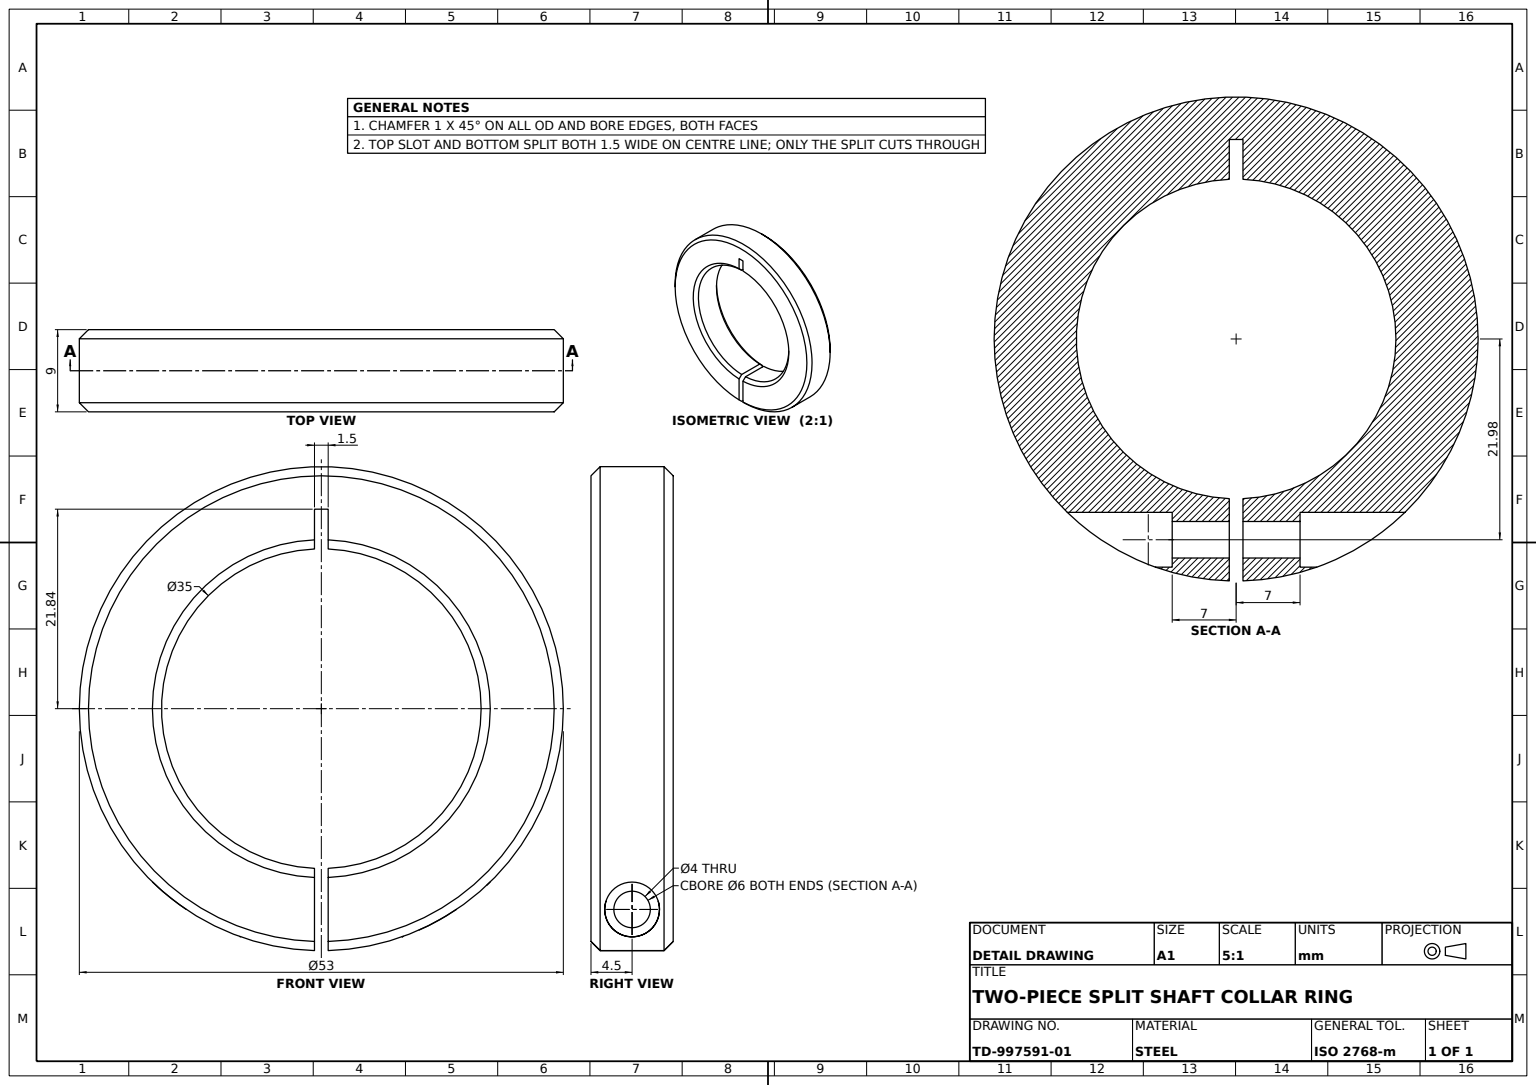
from build123d import *

# Parameters (mm, degrees)
RING_BODY_DEPTH       = 4.5
EDGE_CHAMFER_1MM_SIZE = 1
RADIAL_CUT_DEPTH      = 38.7458607
RADIAL_CUT_DEPTH_BACK = 38.7458607
RADIAL_CUT_SKETCH_R   = 2
SLOT_START            = 7
SLOT_SKETCH_R         = 3
SLOT_CUT_DEPTH        = 25


with BuildPart() as part:
    # Ring Profile Sketch → Ring Body (new, symmetric)
    with BuildSketch(Plane.XY):
        with BuildLine():
            Line((-0.75, 17.483921185), (-0.75, 21.843890817))
            Line((-0.75, 21.843890817), (0.75, 21.843890817))
            Line((0.75, 21.843890817), (0.75, 17.483921185))
            ThreePointArc((0.75, 17.483921185), (17.5, 0), (0.75, -17.483921185))
            Line((0.75, -17.483921185), (0.75, -26.489384666))
            ThreePointArc((0.75, -26.489384666), (0, 26.5), (-0.75, -26.489384666))
            Line((-0.75, -26.489384666), (-0.75, -17.483921185))
            ThreePointArc((-0.75, -17.483921185), (-17.5, 0), (-0.75, 17.483921185))
        make_face()
    extrude(amount=RING_BODY_DEPTH, both=True)

    # Edge Chamfer 1mm
    edge_chamfer_1mm_edges = [part.edges().sort_by_distance(p)[0] for p in [
        (-17.5, 0, -4.5),
        (17.5, 0, 4.5),
        (0, 26.5, 4.5),
        (-17.5, 0, 4.5),
        (0, 26.5, -4.5),
        (17.5, 0, -4.5),
    ]]
    chamfer(edge_chamfer_1mm_edges, length=EDGE_CHAMFER_1MM_SIZE)

    # Radial Cut Sketch → Radial Cut (cut, two sides: drawn at the far end of the back side and taken through both)
    with BuildSketch(Plane(origin=(0, 0, 0), x_dir=(0, 0, -1), z_dir=(1, 0, 0)).offset(-RADIAL_CUT_DEPTH_BACK)):
        with Locations((0, -21.983921185)):
            Circle(RADIAL_CUT_SKETCH_R)
    extrude(amount=RADIAL_CUT_DEPTH + RADIAL_CUT_DEPTH_BACK, mode=Mode.SUBTRACT)

    # Slot Sketch → Slot Cut (cut)
    with BuildSketch(Plane(origin=(0, 0, 0), x_dir=(0, 0, -1), z_dir=(1, 0, 0)).offset(SLOT_START)):
        with Locations(Location((0, -21.983921185, 0), (0, 0, 180))):
            Circle(SLOT_SKETCH_R)
    slot_cut = extrude(amount=SLOT_CUT_DEPTH, mode=Mode.SUBTRACT)

    # Slot Mirror: Slot Cut across plane
    add(slot_cut.mirror(Plane(origin=(0, 0, 0), x_dir=(0, 0, 1), z_dir=(1, 0, 0))), mode=Mode.SUBTRACT)


solid = part.part
